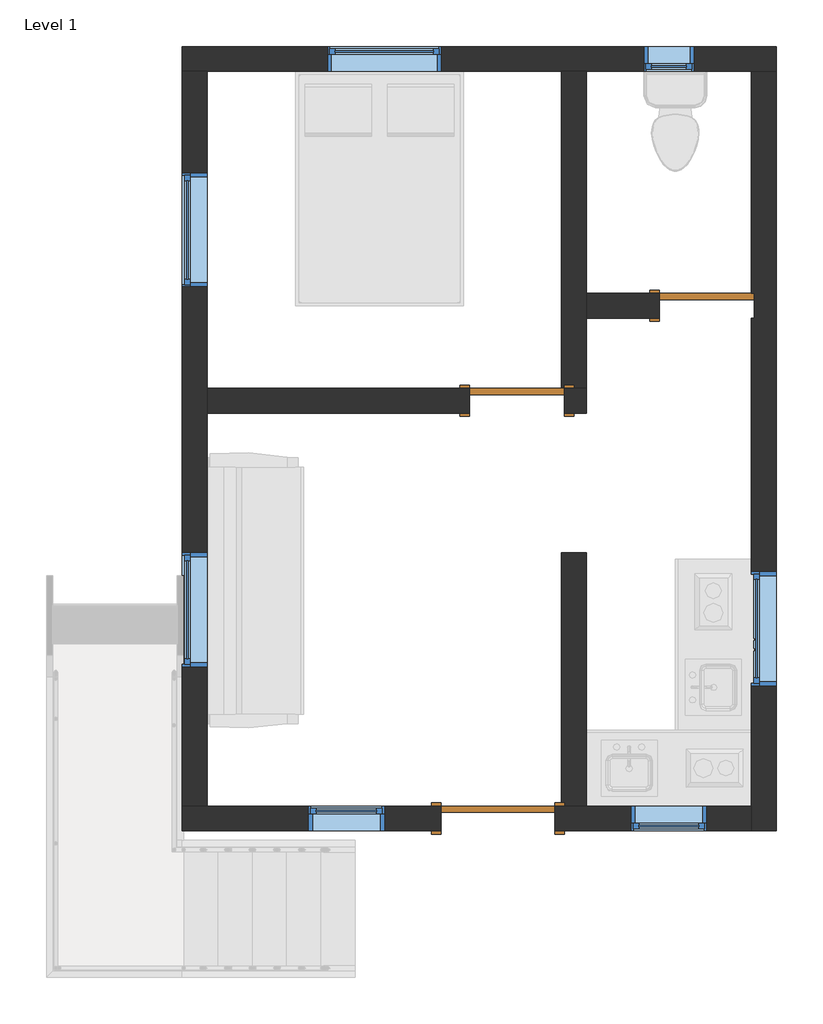
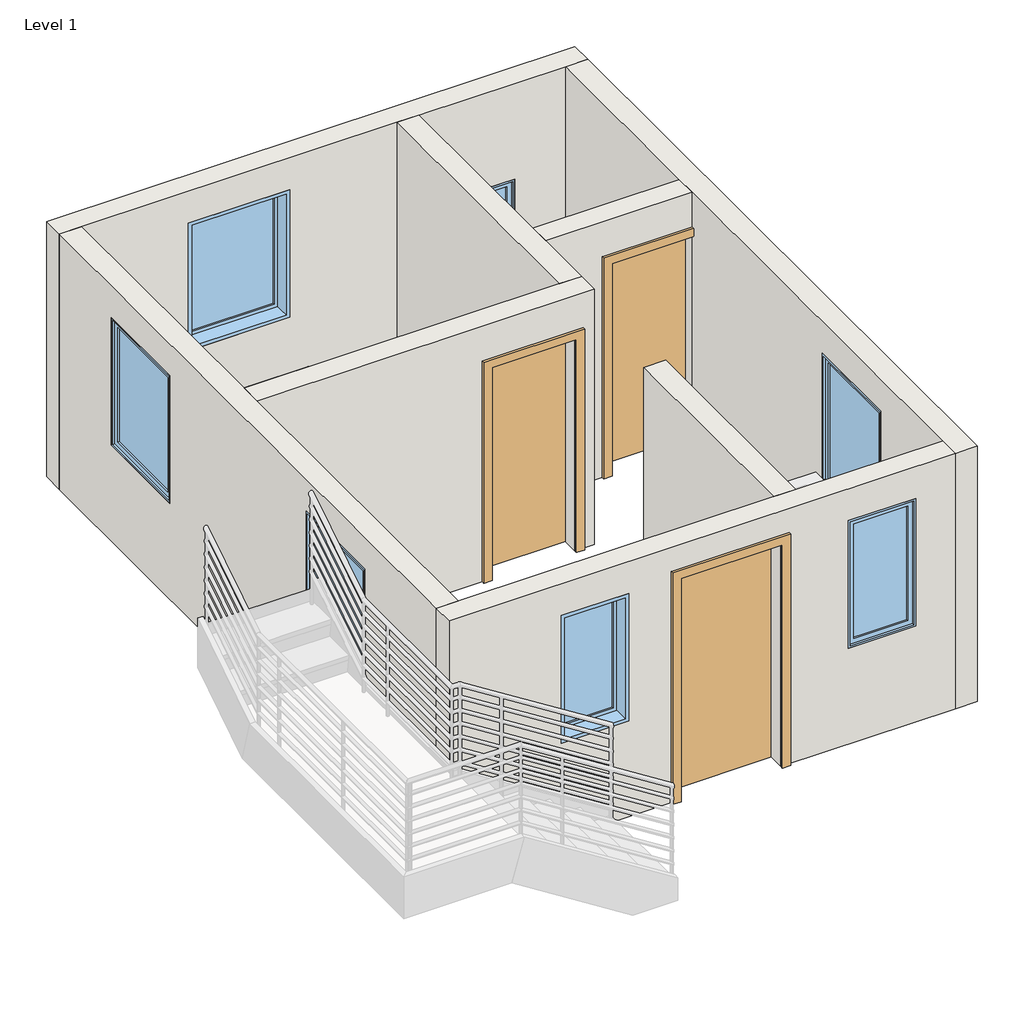
# One storey, part 1 of 3: 8 walls, 7 windows, 3 doors.
"""IFC4 building model written with IfcOpenShell, lengths in millimetres."""

from ifc_helpers import new_model, si_unit, frame, origin, origin_with_axes, place, context, project, spatial, polyline, outline, extrude, faceted_brep, transform, mapped, element, save
from components import m_single_flush_0762_x_2032mm_0c256fab, m_single_flush_0915_x_2134mm_6a9e8738, m_fixed_0406_x_0610mm_8205b201, m_fixed_0610_x_1220mm_4e981104, m_fixed_0915_x_1220mm_488fb2fb, m_fixed_0915_x_1830mm_5d6e8bc1

model = new_model("IFC4")

# Units and contexts
model_context = context("Model", 3, world=origin())
ifc_project = project(units=[si_unit("LENGTHUNIT", "METRE", prefix="MILLI")], contexts=[model_context])

# Site, building, storey
site = spatial("IfcSite", under=ifc_project)
building = spatial("IfcBuilding", under=site)
storey = spatial("IfcBuildingStorey", under=building, Name="Level 1", Elevation=0.0)

# Doors
placement = place(None, origin())
m_single_flush_0762_x_2032mm_shape = m_single_flush_0762_x_2032mm_0c256fab(model_context)
element("IfcDoor", 1, ObjectType="M_Single-Flush : 0762 x 2032mm", at=placement, inside=storey, context=model_context, shape_type="MappedRepresentation", body=[
    mapped(m_single_flush_0762_x_2032mm_shape, transform((-8872.7486562, 9288.0835626, 0.0), x_axis=(1.0, 0.0, 0.0), y_axis=(0.0, 1.0, 0.0), z_axis=(0.0, 0.0, 1.0))),
])
element("IfcDoor", 2, ObjectType="M_Single-Flush : 0762 x 2032mm", at=placement, inside=storey, context=model_context, shape_type="MappedRepresentation", body=[
    mapped(m_single_flush_0762_x_2032mm_shape, transform((-7348.7486562, 10050.0835626, 0.0), x_axis=(1.0, 0.0, 0.0), y_axis=(0.0, 1.0, 0.0), z_axis=(0.0, 0.0, 1.0))),
])
m_single_flush_0915_x_2134mm_shape = m_single_flush_0915_x_2134mm_6a9e8738(model_context)
element("IfcDoor", 3, ObjectType="M_Single-Flush : 0915 x 2134mm", at=placement, inside=storey, context=model_context, shape_type="MappedRepresentation", body=[
    mapped(m_single_flush_0915_x_2134mm_shape, transform((-9025.1486562, 5935.2835626, 0.0), x_axis=(1.0, 0.0, 0.0), y_axis=(0.0, 1.0, 0.0), z_axis=(0.0, 0.0, 1.0))),
])

# Walls
element("IfcWall", 4, ObjectType="Generic - 200mm", at=placement, inside=storey, context=model_context, shape_type="Brep", body=[
    faceted_brep([(-11563.5486562, 11931.2835626, 0.0), (-11363.5486562, 11931.2835626, 0.0), (-8515.5486562, 11931.2835626, 0.0), (-8315.5486562, 11931.2835626, 0.0), (-6991.5486562, 11931.2835626, 0.0), (-6791.5486562, 11931.2835626, 0.0), (-6791.5486562, 11931.2835626, 2438.4), (-6991.5486562, 11931.2835626, 2438.4), (-8315.5486562, 11931.2835626, 2438.4), (-8515.5486562, 11931.2835626, 2438.4), (-11363.5486562, 11931.2835626, 2438.4), (-11563.5486562, 11931.2835626, 2438.4), (-10397.0486562, 11931.2835626, 915.0), (-10397.0486562, 11931.2835626, 2135.0), (-9482.0486562, 11931.2835626, 2135.0), (-9482.0486562, 11931.2835626, 915.0), (-7450.5486562, 11931.2835626, 915.0), (-7856.5486562, 11931.2835626, 915.0), (-7856.5486562, 11931.2835626, 1525.0), (-7450.5486562, 11931.2835626, 1525.0), (-11563.5486562, 12131.2835626, 0.0), (-11563.5486562, 12131.2835626, 2438.4), (-6791.5486562, 12131.2835626, 2438.4), (-6791.5486562, 12131.2835626, 0.0), (-10397.0486562, 12131.2835626, 915.0), (-9482.0486562, 12131.2835626, 915.0), (-9482.0486562, 12131.2835626, 2135.0), (-10397.0486562, 12131.2835626, 2135.0), (-7450.5486562, 12131.2835626, 915.0), (-7450.5486562, 12131.2835626, 1525.0), (-7856.5486562, 12131.2835626, 1525.0), (-7856.5486562, 12131.2835626, 915.0)], [[[0, 1, 2, 3, 4, 5, 6, 7, 8, 9, 10, 11], [12, 13, 14, 15], [16, 17, 18, 19]], [[20, 21, 22, 23], [24, 25, 26, 27], [28, 29, 30, 31]], [[5, 4, 3, 2, 1, 0, 20, 23]], [[11, 10, 9, 8, 7, 6, 22, 21]], [[6, 5, 23, 22]], [[0, 11, 21, 20]], [[13, 12, 24, 27]], [[14, 13, 27, 26]], [[15, 14, 26, 25]], [[12, 15, 25, 24]], [[29, 28, 16, 19]], [[30, 29, 19, 18]], [[31, 30, 18, 17]], [[28, 31, 17, 16]]]),
])
element("IfcWall", 5, ObjectType="Generic - 200mm", at=placement, inside=storey, context=model_context, shape_type="Brep", body=[
    faceted_brep([(-6991.5486562, 5835.2835626, 2438.4), (-6991.5486562, 6035.2835626, 2438.4), (-6991.5486562, 9950.0835626, 2438.4), (-6991.5486562, 10150.0835626, 2438.4), (-6991.5486562, 11931.2835626, 2438.4), (-6991.5486562, 11931.2835626, 0.0), (-6991.5486562, 10150.0835626, 0.0), (-6991.5486562, 10150.0835626, 2032.0), (-6991.5486562, 9950.0835626, 2032.0), (-6991.5486562, 9950.0835626, 0.0), (-6991.5486562, 6035.2835626, 0.0), (-6991.5486562, 5835.2835626, 0.0), (-6991.5486562, 7001.7835626, 305.0), (-6991.5486562, 7916.7835626, 305.0), (-6991.5486562, 7916.7835626, 2135.0), (-6991.5486562, 7001.7835626, 2135.0), (-6791.5486562, 5835.2835626, 0.0), (-6791.5486562, 11931.2835626, 0.0), (-6791.5486562, 11931.2835626, 2438.4), (-6791.5486562, 5835.2835626, 2438.4), (-6791.5486562, 7001.7835626, 305.0), (-6791.5486562, 7001.7835626, 2135.0), (-6791.5486562, 7916.7835626, 2135.0), (-6791.5486562, 7916.7835626, 305.0), (-6967.7486562, 9950.0835626, 0.0), (-6967.7486562, 10150.0835626, 0.0), (-6967.7486562, 9950.0835626, 2032.0), (-6967.7486562, 10150.0835626, 2032.0)], [[[0, 1, 2, 3, 4, 5, 6, 7, 8, 9, 10, 11], [12, 13, 14, 15]], [[16, 17, 18, 19], [20, 21, 22, 23]], [[17, 16, 11, 10, 9, 24, 25, 6, 5]], [[4, 3, 2, 1, 0, 19, 18]], [[5, 4, 18, 17]], [[0, 11, 16, 19]], [[21, 20, 12, 15]], [[22, 21, 15, 14]], [[23, 22, 14, 13]], [[20, 23, 13, 12]], [[26, 24, 9, 8]], [[25, 27, 7, 6]], [[24, 26, 27, 25]], [[27, 26, 8, 7]]]),
])
element("IfcWall", 6, ObjectType="Generic - 200mm", at=placement, inside=storey, context=model_context, shape_type="Brep", body=[
    faceted_brep([(-6991.5486562, 6035.2835626, 0.0), (-8315.5486562, 6035.2835626, 0.0), (-8515.5486562, 6035.2835626, 0.0), (-8567.6486562, 6035.2835626, 0.0), (-8567.6486562, 6035.2835626, 2134.0), (-9482.6486562, 6035.2835626, 2134.0), (-9482.6486562, 6035.2835626, 0.0), (-11363.5486562, 6035.2835626, 0.0), (-11563.5486562, 6035.2835626, 0.0), (-11563.5486562, 6035.2835626, 2438.4), (-11363.5486562, 6035.2835626, 2438.4), (-8515.5486562, 6035.2835626, 2438.4), (-8315.5486562, 6035.2835626, 2438.4), (-6991.5486562, 6035.2835626, 2438.4), (-10549.3486562, 6035.2835626, 915.0), (-9939.3486562, 6035.2835626, 915.0), (-9939.3486562, 6035.2835626, 2135.0), (-10549.3486562, 6035.2835626, 2135.0), (-7348.5486562, 6035.2835626, 915.0), (-7348.5486562, 6035.2835626, 2135.0), (-7958.5486562, 6035.2835626, 2135.0), (-7958.5486562, 6035.2835626, 915.0), (-8567.6486562, 5835.2835626, 2134.0), (-8567.6486562, 5835.2835626, 0.0), (-6991.5486562, 5835.2835626, 0.0), (-6991.5486562, 5835.2835626, 2438.4), (-11563.5486562, 5835.2835626, 2438.4), (-11563.5486562, 5835.2835626, 0.0), (-9482.6486562, 5835.2835626, 0.0), (-9482.6486562, 5835.2835626, 2134.0), (-10549.3486562, 5835.2835626, 915.0), (-10549.3486562, 5835.2835626, 2135.0), (-9939.3486562, 5835.2835626, 2135.0), (-9939.3486562, 5835.2835626, 915.0), (-7348.5486562, 5835.2835626, 915.0), (-7958.5486562, 5835.2835626, 915.0), (-7958.5486562, 5835.2835626, 2135.0), (-7348.5486562, 5835.2835626, 2135.0)], [[[0, 1, 2, 3, 4, 5, 6, 7, 8, 9, 10, 11, 12, 13], [14, 15, 16, 17], [18, 19, 20, 21]], [[22, 23, 24, 25, 26, 27, 28, 29], [30, 31, 32, 33], [34, 35, 36, 37]], [[28, 27, 8, 7, 6]], [[24, 23, 3, 2, 1, 0]], [[13, 12, 11, 10, 9, 26, 25]], [[0, 13, 25, 24]], [[9, 8, 27, 26]], [[31, 30, 14, 17]], [[32, 31, 17, 16]], [[33, 32, 16, 15]], [[30, 33, 15, 14]], [[19, 18, 34, 37]], [[20, 19, 37, 36]], [[21, 20, 36, 35]], [[18, 21, 35, 34]], [[4, 3, 23, 22]], [[5, 4, 22, 29]], [[6, 5, 29, 28]]]),
])
element("IfcWall", 7, ObjectType="Generic - 200mm", at=placement, inside=storey, context=model_context, shape_type="Brep", body=[
    faceted_brep([(-11363.5486562, 6035.2835626, 0.0), (-11363.5486562, 9188.0835626, 0.0), (-11363.5486562, 9388.0835626, 0.0), (-11363.5486562, 11931.2835626, 0.0), (-11363.5486562, 11931.2835626, 2438.4), (-11363.5486562, 9388.0835626, 2438.4), (-11363.5486562, 9188.0835626, 2438.4), (-11363.5486562, 6035.2835626, 2438.4), (-11363.5486562, 10202.1835626, 915.0), (-11363.5486562, 10202.1835626, 2135.0), (-11363.5486562, 11117.1835626, 2135.0), (-11363.5486562, 11117.1835626, 915.0), (-11363.5486562, 7154.1835626, 915.0), (-11363.5486562, 7154.1835626, 2135.0), (-11363.5486562, 8069.1835626, 2135.0), (-11363.5486562, 8069.1835626, 915.0), (-11563.5486562, 6035.2835626, 0.0), (-11563.5486562, 6035.2835626, 2438.4), (-11563.5486562, 11931.2835626, 2438.4), (-11563.5486562, 11931.2835626, 0.0), (-11563.5486562, 10202.1835626, 915.0), (-11563.5486562, 11117.1835626, 915.0), (-11563.5486562, 11117.1835626, 2135.0), (-11563.5486562, 10202.1835626, 2135.0), (-11563.5486562, 7154.1835626, 915.0), (-11563.5486562, 8069.1835626, 915.0), (-11563.5486562, 8069.1835626, 2135.0), (-11563.5486562, 7154.1835626, 2135.0)], [[[0, 1, 2, 3, 4, 5, 6, 7], [8, 9, 10, 11], [12, 13, 14, 15]], [[16, 17, 18, 19], [20, 21, 22, 23], [24, 25, 26, 27]], [[3, 2, 1, 0, 16, 19]], [[7, 6, 5, 4, 18, 17]], [[4, 3, 19, 18]], [[0, 7, 17, 16]], [[9, 8, 20, 23]], [[10, 9, 23, 22]], [[11, 10, 22, 21]], [[8, 11, 21, 20]], [[13, 12, 24, 27]], [[14, 13, 27, 26]], [[15, 14, 26, 25]], [[12, 15, 25, 24]]]),
])
element("IfcWall", 8, ObjectType="Generic - 200mm", at=placement, inside=storey, context=model_context, shape_type="Brep", body=[
    faceted_brep([(-8491.7486562, 9188.0835626, 2032.0), (-8491.7486562, 9188.0835626, 0.0), (-8315.5486562, 9188.0835626, 0.0), (-8315.5486562, 9188.0835626, 2438.4), (-11363.5486562, 9188.0835626, 2438.4), (-11363.5486562, 9188.0835626, 0.0), (-9253.7486562, 9188.0835626, 0.0), (-9253.7486562, 9188.0835626, 2032.0), (-8315.5486562, 9388.0835626, 0.0), (-8491.7486562, 9388.0835626, 0.0), (-8491.7486562, 9388.0835626, 2032.0), (-9253.7486562, 9388.0835626, 2032.0), (-9253.7486562, 9388.0835626, 0.0), (-11363.5486562, 9388.0835626, 0.0), (-11363.5486562, 9388.0835626, 2438.4), (-8515.5486562, 9388.0835626, 2438.4), (-8315.5486562, 9388.0835626, 2438.4)], [[[0, 1, 2, 3, 4, 5, 6, 7]], [[8, 9, 10, 11, 12, 13, 14, 15, 16]], [[6, 5, 13, 12]], [[2, 1, 9, 8]], [[4, 3, 16, 15, 14]], [[5, 4, 14, 13]], [[3, 2, 8, 16]], [[10, 9, 1, 0]], [[11, 10, 0, 7]], [[12, 11, 7, 6]]]),
])
element("IfcWall", 9, ObjectType="Generic - 200mm", at=placement, inside=storey, context=model_context, shape_type="Brep", body=[
    faceted_brep([(-8315.5486562, 9388.0835626, 0.0), (-8315.5486562, 9950.0835626, 0.0), (-8315.5486562, 10150.0835626, 0.0), (-8315.5486562, 11931.2835626, 0.0), (-8315.5486562, 11931.2835626, 2438.4), (-8315.5486562, 10150.0835626, 2438.4), (-8315.5486562, 9950.0835626, 2438.4), (-8315.5486562, 9388.0835626, 2438.4), (-8515.5486562, 9388.0835626, 0.0), (-8515.5486562, 9388.0835626, 2438.4), (-8515.5486562, 11931.2835626, 2438.4), (-8515.5486562, 11931.2835626, 0.0), (-8491.7486562, 9388.0835626, 0.0)], [[[0, 1, 2, 3, 4, 5, 6, 7]], [[8, 9, 10, 11]], [[3, 2, 1, 0, 12, 8, 11]], [[7, 6, 5, 4, 10, 9]], [[0, 7, 9, 8, 12]], [[4, 3, 11, 10]]]),
])
element("IfcWall", 10, ObjectType="Generic - 200mm", at=placement, inside=storey, context=model_context, shape_type="SweptSolid", body=[
    extrude(outline(polyline([(2438.4, -6991.5486562), (2438.4, -8315.5486562), (0.0, -8315.5486562), (0.0, -7729.7486562), (2032.0, -7729.7486562), (2032.0, -6991.5486562), (2438.4, -6991.5486562)])), frame((0.0, 9950.0835626, 0.0), z_axis=(0.0, 1.0, 0.0), x_axis=(0.0, 0.0, 1.0)), (0.0, 0.0, 1.0), 200.0),
])
element("IfcWall", 11, ObjectType="Generic - 200mm", at=placement, inside=storey, context=model_context, shape_type="SweptSolid", body=[
    extrude(outline(polyline([(-8315.5486562, 8068.8835626), (-8315.5486562, 6035.2835626), (-8515.5486562, 6035.2835626), (-8515.5486562, 8068.8835626), (-8315.5486562, 8068.8835626)])), origin_with_axes(), (0.0, 0.0, 1.0), 2438.4),
])

# Windows
m_fixed_0406_x_0610mm_shape = m_fixed_0406_x_0610mm_8205b201(model_context)
element("IfcWindow", 12, ObjectType="M_Fixed : 0406 x 0610mm", at=placement, inside=storey, context=model_context, shape_type="MappedRepresentation", body=[
    mapped(m_fixed_0406_x_0610mm_shape, transform((-7653.5486562, 12044.2835626, 0.0), x_axis=(-1.0, 0.0, 0.0), y_axis=(0.0, -1.0, 0.0), z_axis=(0.0, 0.0, 1.0))),
])
m_fixed_0610_x_1220mm_shape = m_fixed_0610_x_1220mm_4e981104(model_context)
element("IfcWindow", 13, ObjectType="M_Fixed : 0610 x 1220mm", at=placement, inside=storey, context=model_context, shape_type="MappedRepresentation", body=[
    mapped(m_fixed_0610_x_1220mm_shape, transform((-10244.3486562, 5922.2835626, 0.0), x_axis=(1.0, 0.0, 0.0), y_axis=(0.0, 1.0, 0.0), z_axis=(0.0, 0.0, 1.0))),
])
element("IfcWindow", 14, ObjectType="M_Fixed : 0610 x 1220mm", at=placement, inside=storey, context=model_context, shape_type="MappedRepresentation", body=[
    mapped(m_fixed_0610_x_1220mm_shape, transform((-7653.5486562, 5948.2835626, 0.0), x_axis=(-1.0, 0.0, 0.0), y_axis=(0.0, -1.0, 0.0), z_axis=(0.0, 0.0, 1.0))),
])
m_fixed_0915_x_1220mm_shape = m_fixed_0915_x_1220mm_488fb2fb(model_context)
element("IfcWindow", 15, ObjectType="M_Fixed : 0915 x 1220mm", at=placement, inside=storey, context=model_context, shape_type="MappedRepresentation", body=[
    mapped(m_fixed_0915_x_1220mm_shape, transform((-11450.5486562, 10659.6835626, 0.0), x_axis=(0.0, 1.0, 0.0), y_axis=(-1.0, 0.0, 0.0), z_axis=(0.0, 0.0, 1.0))),
])
element("IfcWindow", 16, ObjectType="M_Fixed : 0915 x 1220mm", at=placement, inside=storey, context=model_context, shape_type="MappedRepresentation", body=[
    mapped(m_fixed_0915_x_1220mm_shape, transform((-9939.5486562, 12018.2835626, 0.0), x_axis=(1.0, 0.0, 0.0), y_axis=(0.0, 1.0, 0.0), z_axis=(0.0, 0.0, 1.0))),
])
element("IfcWindow", 17, ObjectType="M_Fixed : 0915 x 1220mm", at=placement, inside=storey, context=model_context, shape_type="MappedRepresentation", body=[
    mapped(m_fixed_0915_x_1220mm_shape, transform((-11450.5486562, 7611.6835626, 0.0), x_axis=(0.0, 1.0, 0.0), y_axis=(-1.0, 0.0, 0.0), z_axis=(0.0, 0.0, 1.0))),
])
m_fixed_0915_x_1830mm_shape = m_fixed_0915_x_1830mm_5d6e8bc1(model_context)
element("IfcWindow", 18, ObjectType="M_Fixed : 0915 x 1830mm", at=placement, inside=storey, context=model_context, shape_type="MappedRepresentation", body=[
    mapped(m_fixed_0915_x_1830mm_shape, transform((-6878.5486562, 7459.2835626, 0.0), x_axis=(0.0, 1.0, 0.0), y_axis=(-1.0, 0.0, 0.0), z_axis=(0.0, 0.0, 1.0))),
])

save(model, "model.ifc")

# Revit data of these elements
# Type "M_Single-Flush : 0762 x 2032mm"
#   Type Mark = "19"
#   Thickness = 51 mm
#   Height = 2032 mm
#   Trim Projection Ext = 25 mm
#   Trim Projection Int = 25 mm
#   Trim Width = 76 mm
#   Width = 762 mm
#   Door Material = Door - Panel
#   Frame Material = Door - Frame
#   Function = (empty or 0)
#   Wall Closure = (empty or 0)
# Type "M_Single-Flush : 0915 x 2134mm"
#   Type Mark = "15"
#   Thickness = 51 mm
#   Height = 2134 mm
#   Trim Projection Ext = 25 mm
#   Trim Projection Int = 25 mm
#   Trim Width = 76 mm
#   Width = 915 mm
#   Door Material = Door - Panel
#   Frame Material = Door - Frame
#   Function = (empty or 0)
#   Wall Closure = (empty or 0)
# Type "Generic - 200mm"
#   Layers, outside or top first: 200 mm no material (function 1)
# Type "M_Fixed : 0406 x 0610mm"
#   Type Mark = "10"
#   Height = 610 mm
#   Default Sill Height = 915 mm
#   Width = 406 mm
#   Window Inset = 19 mm
#   Frame Exterior Material = Sash
#   Frame Interior Material = Sash
#   Glass Pane Material = Glass
#   Sash = Sash
#   Wall Closure = (empty or 0)
# Type "M_Fixed : 0610 x 1220mm"
#   Type Mark = "13"
#   Height = 1220 mm
#   Default Sill Height = 915 mm
#   Width = 610 mm
#   Window Inset = 19 mm
#   Frame Exterior Material = Sash
#   Frame Interior Material = Sash
#   Glass Pane Material = Glass
#   Sash = Sash
#   Wall Closure = (empty or 0)
# Type "M_Fixed : 0915 x 1220mm"
#   Type Mark = "15"
#   Height = 1220 mm
#   Default Sill Height = 915 mm
#   Width = 915 mm
#   Window Inset = 19 mm
#   Frame Exterior Material = Sash
#   Frame Interior Material = Sash
#   Glass Pane Material = Glass
#   Sash = Sash
#   Wall Closure = (empty or 0)
# Type "M_Fixed : 0915 x 1830mm"
#   Type Mark = "18"
#   Height = 1830 mm
#   Default Sill Height = 305 mm
#   Width = 915 mm
#   Window Inset = 19 mm
#   Frame Exterior Material = Sash
#   Frame Interior Material = Sash
#   Glass Pane Material = Glass
#   Sash = Sash
#   Wall Closure = (empty or 0)
# Elements 1, 2 (IfcDoor, "M_Single-Flush : 0762 x 2032mm")
#   Phase Created = New Construction
#   Materials on its faces: "Door - Frame", "Door - Panel"
# Element 3 (IfcDoor, "M_Single-Flush : 0915 x 2134mm")
#   Phase Created = New Construction
#   Materials on its faces: "Door - Frame", "Door - Panel"
# Elements 4, 5, 6, 7, 8, 9, 10, 11 (IfcWall, "Generic - 200mm")
#   Top Offset = 0 mm
#   Base Offset = 0 mm
#   Unconnected Height = 2438.4 mm
#   wall height = 2438.4 mm
#   Phase Created = New Construction
#   Base Constraint = Level 1
#   Materials on its faces: "Default Wall"
# Element 12 (IfcWindow, "M_Fixed : 0406 x 0610mm")
#   Mark = "12"
#   Phase Created = New Construction
#   Materials on its faces: "Sash", "Glass"
# Element 13 (IfcWindow, "M_Fixed : 0610 x 1220mm")
#   Mark = "9"
#   Phase Created = New Construction
#   Materials on its faces: "Sash", "Glass"
# Element 14 (IfcWindow, "M_Fixed : 0610 x 1220mm")
#   Mark = "10"
#   Phase Created = New Construction
#   Materials on its faces: "Sash", "Glass"
# Element 15 (IfcWindow, "M_Fixed : 0915 x 1220mm")
#   Mark = "6"
#   Phase Created = New Construction
#   Materials on its faces: "Sash", "Glass"
# Element 16 (IfcWindow, "M_Fixed : 0915 x 1220mm")
#   Mark = "7"
#   Phase Created = New Construction
#   Materials on its faces: "Sash", "Glass"
# Element 17 (IfcWindow, "M_Fixed : 0915 x 1220mm")
#   Mark = "8"
#   Phase Created = New Construction
#   Materials on its faces: "Sash", "Glass"
# Element 18 (IfcWindow, "M_Fixed : 0915 x 1830mm")
#   Mark = "11"
#   Phase Created = New Construction
#   Materials on its faces: "Sash", "Glass"
# Materials
#   "Door - Panel": class "Wood", colour RGB 114 82 51, transparency 0
#   "Door - Frame": colour RGB 153 76 43, transparency 0
#   "Sash": class "Wood", colour RGB 136 99 55, transparency 0
#   "Glass": class "Glass", colour RGB 218 227 224, transparency 0.85, Description = "Soda Lime Glass", Cost = 0
#   "Default Wall": colour RGB 80 80 80, transparency 0
